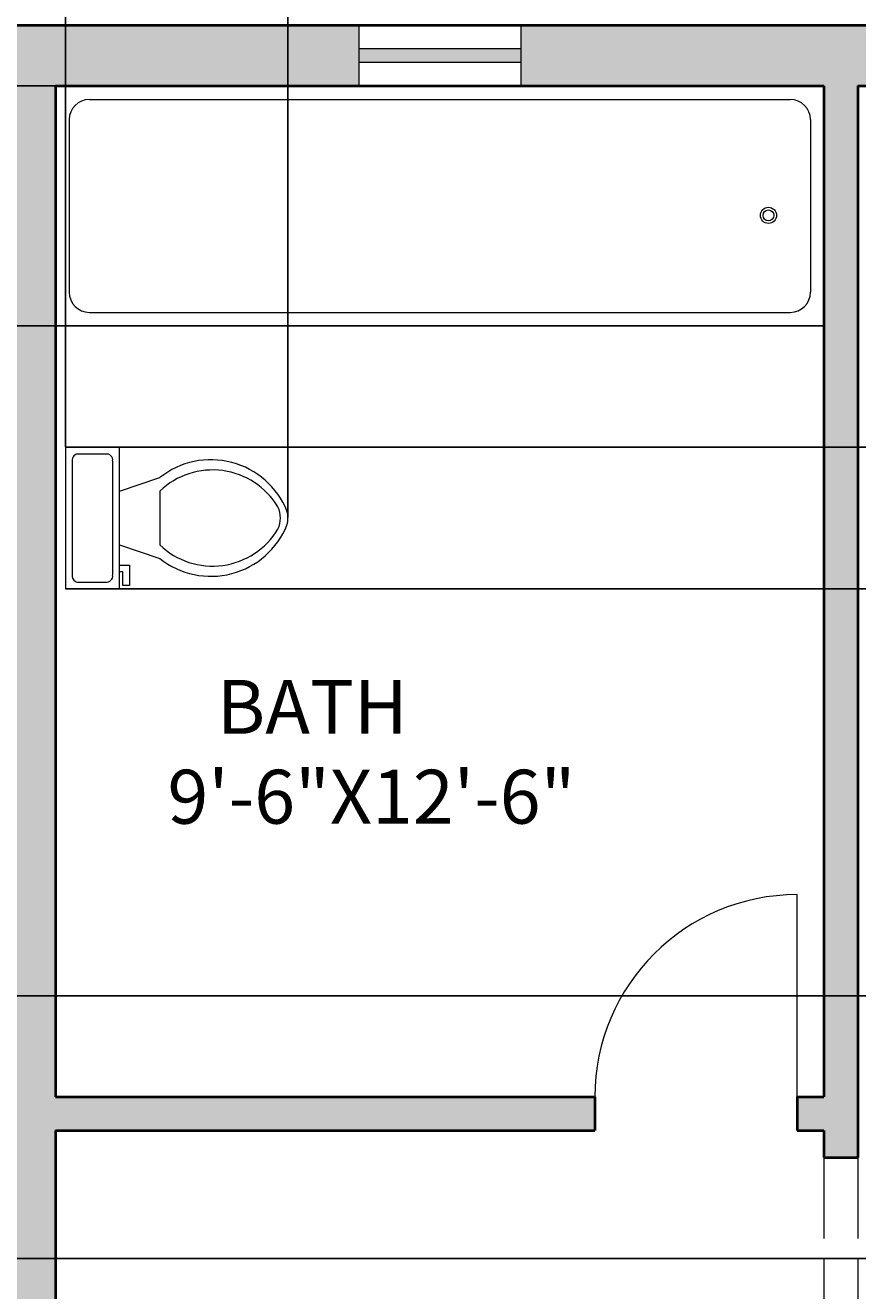
# Model space of a CAD drawing. Units: inches. Extents: x 2330 to 3943, y 1763 to 3461.
# Tile 27 of 40: x 2973 to 3097, y 2975 to 3163. Entities that reach past the tile are written whole.
import ezdxf

# ---------------------------------------------------------------- set-up
doc = ezdxf.new("R2010")
doc.units = ezdxf.units.IN
doc.linetypes.add('ACAD_ISO02W100', pattern=[15, 12, -3])
for name, color, linetype, lineweight in [('A-ANNO-DIMS', 2, 'Continuous', 18), ('A-AREA-IDEN', 7, 'Continuous', 18), ('A-DOOR', 4, 'Continuous', 18), ('A-FLOR-FIXT', 8, 'Continuous', 18), ('A-GLAZ', 4, 'Continuous', 18), ('A-WALL', 7, 'Continuous', 40), ('A-WALL-OVHD', 7, 'ACAD_ISO02W100', 18), ('A-WALL-PATT', 252, 'Continuous', 13)]:
    doc.layers.add(name, color=color, linetype=linetype, lineweight=lineweight)
doc.styles.get("Standard").update_dxf_attribs({"font": 'arial.ttf'})
doc.dimstyles.get("Standard").update_dxf_attribs({"dimtxt": 0.18, "dimasz": 0.18, "dimexe": 0.18, "dimexo": 0.0625, "dimgap": 0.09, "dimtad": 0, "dimtih": 1, "dimtoh": 1, "dimdec": 4, "dimzin": 0, "dimdsep": 46, "dimtxsty": 'Standard', "dimcen": 0.09, "dimadec": 0, "dimazin": 0, "dimtfac": 1, "dimtdec": 4, "dimtofl": 0, "dimtmove": 0, "dimatfit": 3, "dimfxl": 1, "dimtolj": 1, "dimtzin": 0, "dimarcsym": 0})

# ---------------------------------------------------------------- blocks, each defined once
blk = doc.blocks.new('*U9')
for p, q in [((9.5, -6), (9.5, -2)), ((-10, -8.5), (-8, -8.5)), ((-10, -9.5), (-10, -8.5)), ((-8, -8.5), (-8, -8)), ((-7, -8), (-7, -9.5)), ((-4, -8), (-6, -14)), ((4, -8), (6, -14)), ((-7, -9.5), (-10, -9.5)), ((4, -14), (-4, -14))]:
    blk.add_line(p, q)
blk.add_lwpolyline([(10.5, -8), (10.5, 0), (-10.5, 0), (-10.5, -8)], close=True)
for points in [[(8.5, -1), (-8.5, -1)], [(-9.5, -2), (-9.5, -6)], [(-8.5, -7), (8.5, -7)]]:
    blk.add_lwpolyline(points)
for centre, radius, start, end in [((-8.62, -1.88), 0.884, 81.8699, 188.1301), ((8.62, -1.88), 0.884, 351.8699, 98.1301), ((-8.62, -6.12), 0.884, 171.8699, 278.1301), ((8.62, -6.12), 0.884, 261.8699, 8.1301), ((3.52, -21.58), 12.17, 141.4691, 247.9714), ((4.2, -21.82), 11.33, 136.3677, 238.9468), ((-3.52, -21.58), 12.17, 292.0284, 38.5307), ((-4.2, -21.82), 11.33, 301.053, 43.6321), ((0, -27.88), 4, 245.7318, 294.2682), ((0, -29), 4, 254.8605, 285.1395)]:
    blk.add_arc(centre, radius, start, end)
blk = doc.blocks.new('DOOR-SINGLE-30IN')
blk.add_line((0, 0), (0, 30))
blk.add_arc((0, 0), 30, 90, 180)
blk = doc.blocks.new('WINDOW-24IN')
h = blk.add_hatch(color=256)
h.dxf.hatch_style = 1
h.paths.add_polyline_path([(5.5, 24), (3.5, 24), (3.5, 0), (5.5, 0)])
for p, q in [((9, 24), (0, 24)), ((3.5, 24), (3.5, 0)), ((5.5, 24), (5.5, 0)), ((9, 0), (0, 0))]:
    blk.add_line(p, q)
blk = doc.blocks.new('*D85')
at = {"layer": 'A-ANNO-DIMS', "color": 0, "lineweight": -2, "transparency": 16777216}
for p, q in [((3091.6, 3153.65), (2330.5, 3153.65)), ((2330.68, 3153.47), (2330.68, 3136.04)), ((2330.68, 3118.24), (2330.68, 3135.67)), ((3091.6, 3118.06), (2330.5, 3118.06))]:
    blk.add_line(p, q, dxfattribs=at)
at = {"layer": 'A-ANNO-DIMS', "color": 0, "transparency": 16777216}
for points in [[(2330.65, 3153.47), (2330.71, 3153.47), (2330.68, 3153.65)], [(2330.65, 3118.24), (2330.71, 3118.24), (2330.68, 3118.06)]]:
    blk.add_solid(points, dxfattribs=at)
at = {"layer": 'Defpoints', "color": 0, "transparency": 16777216}
for p in [(2330.68, 3153.65), (3091.66, 3153.65), (3091.66, 3118.06)]:
    blk.add_point(p, dxfattribs=at)
at = {"layer": 'A-ANNO-DIMS', "color": 0, "transparency": 16777216, "insert": (2330.68, 3135.86), "char_height": 0.18, "attachment_point": 5}
blk.add_mtext('\\A1;35.59', dxfattribs=at)
blk = doc.blocks.new('*D86')
at = {"layer": 'A-ANNO-DIMS', "color": 0, "lineweight": -2, "transparency": 16777216}
for p, q in [((2979.18, 3100.04), (3942.54, 3100.04)), ((3942.36, 3099.86), (3942.36, 3089.72)), ((3942.36, 3079.22), (3942.36, 3089.36)), ((2979.18, 3079.04), (3942.54, 3079.04))]:
    blk.add_line(p, q, dxfattribs=at)
at = {"layer": 'A-ANNO-DIMS', "color": 0, "transparency": 16777216}
for points in [[(3942.33, 3099.86), (3942.39, 3099.86), (3942.36, 3100.04)], [(3942.33, 3079.22), (3942.39, 3079.22), (3942.36, 3079.04)]]:
    blk.add_solid(points, dxfattribs=at)
at = {"layer": 'Defpoints', "color": 0, "transparency": 16777216}
for p in [(2979.12, 3100.04), (2979.12, 3079.04), (3942.36, 3079.04)]:
    blk.add_point(p, dxfattribs=at)
at = {"layer": 'A-ANNO-DIMS', "color": 0, "transparency": 16777216, "insert": (3942.36, 3089.54), "char_height": 0.18, "attachment_point": 5}
blk.add_mtext('\\A1;21', dxfattribs=at)
blk = doc.blocks.new('*D87')
at = {"layer": 'A-ANNO-DIMS', "color": 0, "lineweight": -2, "transparency": 16777216}
for p, q in [((2979.12, 3100.1), (2979.12, 3461.3)), ((2979.3, 3461.12), (2995.4, 3461.12)), ((3011.94, 3461.12), (2995.84, 3461.12)), ((3012.12, 3089.6), (3012.12, 3461.3))]:
    blk.add_line(p, q, dxfattribs=at)
at = {"layer": 'A-ANNO-DIMS', "color": 0, "transparency": 16777216}
for points in [[(2979.3, 3461.15), (2979.3, 3461.09), (2979.12, 3461.12)], [(3011.94, 3461.15), (3011.94, 3461.09), (3012.12, 3461.12)]]:
    blk.add_solid(points, dxfattribs=at)
at = {"layer": 'Defpoints', "color": 0, "transparency": 16777216}
for p in [(3012.12, 3461.12), (2979.12, 3100.04), (3012.12, 3089.54)]:
    blk.add_point(p, dxfattribs=at)
at = {"layer": 'A-ANNO-DIMS', "color": 0, "transparency": 16777216, "insert": (2995.62, 3461.12), "char_height": 0.18, "attachment_point": 5}
blk.add_mtext('\\A1;33', dxfattribs=at)
blk = doc.blocks.new('*D93')
at = {"layer": 'A-ANNO-DIMS', "color": 0, "lineweight": -2, "transparency": 16777216}
for p, q in [((3446.6, 3018.65), (2330.5, 3018.65)), ((2330.68, 3018.47), (2330.68, 2999.33)), ((2330.68, 2979.83), (2330.68, 2998.97)), ((3446.6, 2979.65), (2330.5, 2979.65))]:
    blk.add_line(p, q, dxfattribs=at)
at = {"layer": 'A-ANNO-DIMS', "color": 0, "transparency": 16777216}
for points in [[(2330.65, 3018.47), (2330.71, 3018.47), (2330.68, 3018.65)], [(2330.65, 2979.83), (2330.71, 2979.83), (2330.68, 2979.65)]]:
    blk.add_solid(points, dxfattribs=at)
at = {"layer": 'Defpoints', "color": 0, "transparency": 16777216}
for p in [(2330.68, 3018.65), (3446.66, 3018.65), (3446.66, 2979.65)]:
    blk.add_point(p, dxfattribs=at)
at = {"layer": 'A-ANNO-DIMS', "color": 0, "transparency": 16777216, "insert": (2330.68, 2999.15), "char_height": 0.18, "attachment_point": 5}
blk.add_mtext('\\A1;39', dxfattribs=at)

msp = doc.modelspace()

# ---------------------------------------------------------------- hatches: boundary and pattern name
at = {"layer": 'A-WALL-PATT'}
h = msp.add_hatch(color=256, dxfattribs=at)
h.dxf.hatch_style = 1
h.paths.add_polyline_path([(3022.6605, 3162.6524), (2968.6605, 3162.6524), (2968.6605, 3083.6524), (2916.6605, 3083.6524), (2916.6605, 3074.6524), (2968.6605, 3074.6524), (2968.6605, 2863.6524), (2977.6605, 2863.6524), (2977.6605, 2867.6524), (3096.6605, 2867.6524), (3096.6605, 2913.1524), (3114.6605, 2913.1524), (3114.6605, 2918.1524), (3096.6605, 2918.1524), (3096.6605, 2958.6524), (3091.6605, 2958.6524), (3091.6605, 2872.6524), (2977.6605, 2872.6524), (2977.6605, 2998.6524), (3057.6605, 2998.6524), (3057.6605, 3003.6524), (2977.6605, 3003.6524), (2977.6605, 3153.6524), (3022.6605, 3153.6524)])
h = msp.add_hatch(color=256, dxfattribs=at)
h.dxf.hatch_style = 1
h.paths.add_polyline_path([(3123.6605, 3162.6524), (3046.6605, 3162.6524), (3046.6605, 3153.6524), (3091.6605, 3153.6524), (3091.6605, 3003.6524), (3087.6605, 3003.6524), (3087.6605, 2998.6524), (3091.6605, 2998.6524), (3091.6605, 2994.6524), (3096.6605, 2994.6524), (3096.6605, 3153.6524), (3123.6605, 3153.6524)])

# ---------------------------------------------------------------- linework, layer by layer
at = {"layer": 'A-FLOR-FIXT'}
for p, q in [((2982.6605, 3151.6524), (3086.6605, 3151.6524)), ((2979.6605, 3148.6524), (2979.6605, 3123.0598)), ((3089.6605, 3148.6524), (3089.6605, 3123.0598)), ((2982.6605, 3120.0598), (3086.6605, 3120.0598)), ((2977.6605, 3118.0598), (3091.6605, 3118.0598))]:
    msp.add_line(p, q, dxfattribs=at)
for radius in [1.197, 0.8065]:
    msp.add_circle((3083.419, 3134.4502), radius, dxfattribs=at)
for centre, start, end in [((2982.6605, 3148.6524), 90, 180), ((3086.6605, 3148.6524), 0, 90), ((2982.6605, 3123.0598), 180, 270), ((3086.6605, 3123.0598), 270, 0)]:
    msp.add_arc(centre, 3, start, end, dxfattribs=at)
at = {"layer": 'A-WALL'}
for p, q in [((2968.6605, 3162.6524), (3455.6605, 3162.6524)), ((2977.6605, 3153.6524), (2977.6605, 3003.6524)), ((2977.6605, 3153.6524), (3091.6605, 3153.6524)), ((3091.6605, 3153.6524), (3091.6605, 3003.6524)), ((3096.6605, 3153.6524), (3096.6605, 2994.6524)), ((3096.6605, 3153.6524), (3270.6605, 3153.6524)), ((2977.6605, 3003.6524), (3057.6605, 3003.6524)), ((3057.6605, 3003.6524), (3057.6605, 2998.6524)), ((3087.6605, 3003.6524), (3087.6605, 2998.6524)), ((3087.6605, 3003.6524), (3091.6605, 3003.6524)), ((2977.6605, 2998.6524), (3057.6605, 2998.6524)), ((2977.6605, 2998.6524), (2977.6605, 2872.6524)), ((3087.6605, 2998.6524), (3091.6605, 2998.6524)), ((3091.6605, 2998.6524), (3091.6605, 2994.6524)), ((3091.6605, 2994.6524), (3096.6605, 2994.6524))]:
    msp.add_line(p, q, dxfattribs=at)
at = {"layer": 'A-WALL-OVHD'}
for p, q in [((3091.6605, 2994.6524), (3091.6605, 2958.6524)), ((3096.6605, 2994.6524), (3096.6605, 2958.6524))]:
    msp.add_line(p, q, dxfattribs=at)

# ---------------------------------------------------------------- block references
at = {"layer": 'A-DOOR'}
msp.add_blockref('DOOR-SINGLE-30IN', (3087.6605, 3003.6524), dxfattribs=at)
at = {"layer": 'A-FLOR-FIXT', "rotation": 90}
msp.add_blockref('*U9', (2979.1218, 3089.5386), dxfattribs=at)
at = {"layer": 'A-GLAZ', "extrusion": (0, 0, -1), "zscale": -1, "rotation": 89.99999999999999}
msp.add_blockref('WINDOW-24IN', (-3022.6605, 3153.6524), dxfattribs=at)

# ---------------------------------------------------------------- texts
at = {"layer": 'A-AREA-IDEN', "insert": (2994.2514, 3065.5199), "char_height": 8, "attachment_point": 1}
msp.add_mtext_dynamic_manual_height_columns('   BATH\\P9\'-6"X12\'-6"', width=89.990069, gutter_width=12.5, heights=[0], dxfattribs=at)

# ---------------------------------------------------------------- dimensions: what is measured, and where the dimension line sits
at = {"layer": 'A-ANNO-DIMS'}
dim = msp.add_linear_dim(base=(3012.1218, 3461.1231), p1=(2979.1218, 3100.0386), p2=(3012.1218, 3089.5386), dimstyle='Standard', override={"dimdec": 0, "dimlfac": 1, "dimrnd": 0, "dimzin": 0, "dimdsep": 46, "dimlunit": 2}, dxfattribs=at)
dim.commit()
dim.dimension.update_dxf_attribs({"geometry": '*D87', "text_midpoint": (2995.6218, 3461.1231)})
for base, p1, p2, override, picture, middle in [((2330.6824, 3153.6524), (3091.6605, 3118.0598), (3091.6605, 3153.6524), {"dimdec": 2, "dimlfac": 1, "dimrnd": 0, "dimzin": 0, "dimdsep": 46, "dimlunit": 2}, '*D85', (2330.6824, 3135.8561)), ((3942.361, 3079.0386), (2979.1218, 3100.0386), (2979.1218, 3079.0386), {"dimdec": 0, "dimlfac": 1, "dimrnd": 0, "dimzin": 0, "dimdsep": 46, "dimlunit": 2}, '*D86', (3942.361, 3089.5386)), ((2330.6824, 3018.6524), (3446.6605, 2979.6524), (3446.6605, 3018.6524), {"dimdec": 0, "dimlfac": 1, "dimrnd": 0, "dimzin": 0, "dimdsep": 46, "dimlunit": 2}, '*D93', (2330.6824, 2999.1524))]:
    dim = msp.add_linear_dim(base=base, p1=p1, p2=p2, angle=90, dimstyle='Standard', override=override, dxfattribs=at)
    dim.commit()
    dim.dimension.update_dxf_attribs({"geometry": picture, "text_midpoint": middle})

doc.saveas('drawing.dxf')
